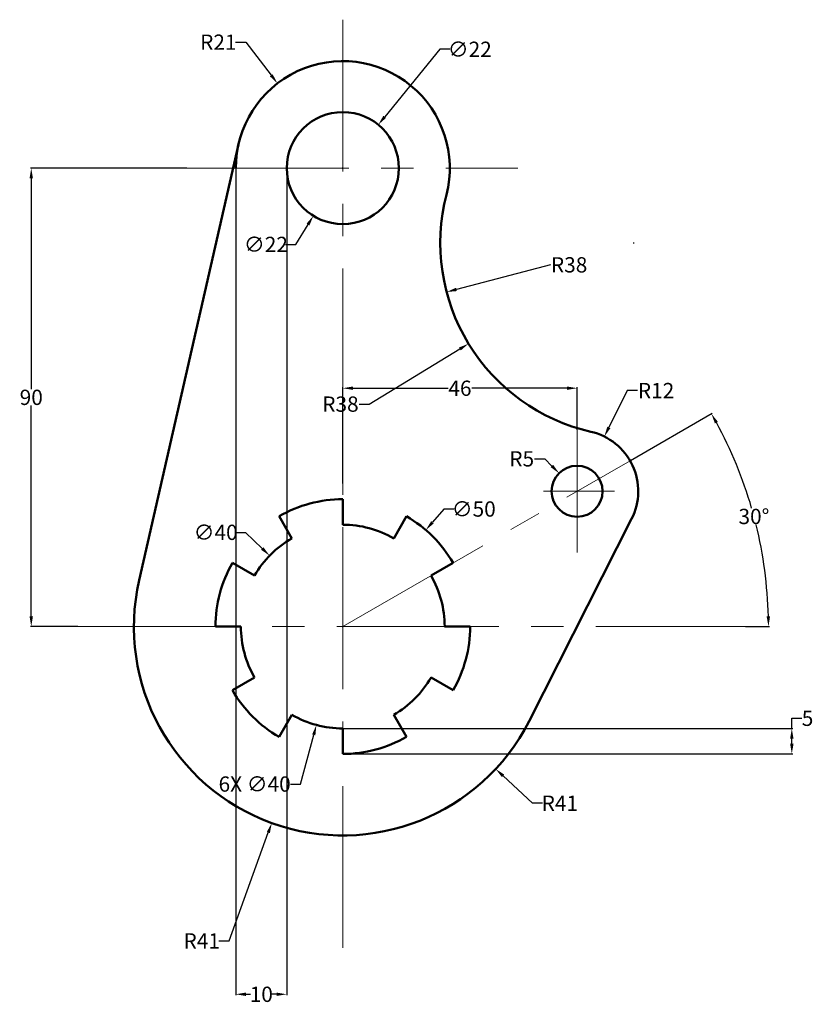
# Model space of a CAD drawing. Units: inches. Extents: x 93 to 249, y 22 to 215.
import ezdxf

# ---------------------------------------------------------------- set-up
doc = ezdxf.new("R2010")
doc.units = ezdxf.units.IN
doc.header["$MEASUREMENT"] = 0
doc.linetypes.add('CENTER', pattern=[50.8, 31.75, -6.35, 6.35, -6.35])
for name, color, linetype, lineweight in [('M-CNTR', 4, 'CENTER', 18), ('M-DIMS', 2, 'Continuous', 25), ('M-OUTL', 7, 'Continuous', 50)]:
    doc.layers.add(name, color=color, linetype=linetype, lineweight=lineweight)
doc.styles.get("Standard").update_dxf_attribs({"font": 'arial.ttf'})
doc.dimstyles.get("Standard").update_dxf_attribs({"dimtxt": 3, "dimasz": 2, "dimexe": 0.18, "dimexo": 0.0625, "dimgap": 0.09, "dimtad": 0, "dimtih": 1, "dimtoh": 1, "dimdec": 0, "dimzin": 0, "dimdsep": 46, "dimtxsty": 'Standard', "dimcen": 0.09, "dimadec": 0, "dimazin": 0, "dimtfac": 1, "dimtdec": 0, "dimtofl": 0, "dimtmove": 0, "dimatfit": 3, "dimfxl": 1, "dimtolj": 1, "dimtzin": 0, "dimarcsym": 0})

# ---------------------------------------------------------------- blocks, each defined once
blk = doc.blocks.new('*U1')
for p, q in [((6.25, -1.16), (6.25, 3.84)), ((-3.75, -3.84), (-6.25, 0.49))]:
    blk.add_line(p, q)
blk.add_arc((6.25, -21.16), 25, 90, 120)
blk = doc.blocks.new('*U2')
at = {"layer": 'M-OUTL', "color": 0, "linetype": 'ByBlock', "lineweight": -2, "transparency": 16777216}
blk.add_blockref('*U1', (150.02, 117.01), dxfattribs=at)
for p, rotation in [((171.47, 111.84), 300), ((134.82, 101.02), 59.99999999999996), ((177.72, 90.68), 239.9999999999999), ((141.07, 79.85), 119.9999999999999), ((162.52, 74.69), 180)]:
    blk.add_blockref('*U1', p, dxfattribs=dict(at, rotation=rotation))
blk = doc.blocks.new('*D3')
at = {"layer": 'Defpoints', "color": 0, "transparency": 16777216}
for p in [(212.66, 128.41), (238.56, 110.36), (104.32, 95.85), (156.27, 95.85), (235.29, 95.85)]:
    blk.add_point(p, dxfattribs=at)
at = {"layer": 'M-DIMS', "color": 0, "lineweight": -2, "transparency": 16777216}
for p, q in [((212.72, 128.44), (228.79, 137.72)), ((235.35, 95.85), (240.01, 95.85))]:
    blk.add_line(p, q, dxfattribs=at)
for start, end in [(16.1552, 28.6286), (1.3714, 13.851)]:
    blk.add_arc((156.27, 95.85), 83.56, start, end, dxfattribs=at)
at = {"layer": 'M-DIMS', "color": 0, "transparency": 16777216}
for points in [[(229.32, 135.72), (229.9, 136.05), (228.63, 137.63)], [(240.14, 97.85), (239.47, 97.84), (239.83, 95.85)]]:
    blk.add_solid(points, dxfattribs=at)
at = {"layer": 'M-DIMS', "color": 0, "transparency": 16777216, "insert": (236.98, 117.47), "char_height": 3, "attachment_point": 5}
blk.add_mtext('\\A1;30°', dxfattribs=at)
blk = doc.blocks.new('*D4')
at = {"layer": 'Defpoints', "color": 0, "transparency": 16777216}
for p in [(207.61, 133.15), (202.27, 122.41)]:
    blk.add_point(p, dxfattribs=at)
at = {"layer": 'M-DIMS', "color": 0, "lineweight": -2, "transparency": 16777216}
for p, q in [((212.1, 142.18), (208.5, 134.94)), ((214.1, 142.18), (212.1, 142.18)), ((202.18, 122.41), (202.36, 122.41)), ((202.27, 122.32), (202.27, 122.5))]:
    blk.add_line(p, q, dxfattribs=at)
at = {"layer": 'M-DIMS', "color": 0, "transparency": 16777216}
blk.add_solid([(208.2, 135.09), (208.8, 134.79), (207.61, 133.15)], dxfattribs=at)
at = {"layer": 'M-DIMS', "color": 0, "transparency": 16777216, "insert": (217.76, 142.18), "char_height": 3, "attachment_point": 5}
blk.add_mtext('\\A1;R12', dxfattribs=at)
blk = doc.blocks.new('*D5')
at = {"layer": 'Defpoints', "color": 0, "transparency": 16777216}
for p in [(198.74, 125.95), (202.27, 122.41)]:
    blk.add_point(p, dxfattribs=at)
at = {"layer": 'M-DIMS', "color": 0, "lineweight": -2, "transparency": 16777216}
for p, q in [((193.91, 128.78), (195.91, 128.78)), ((195.91, 128.78), (197.33, 127.36)), ((202.18, 122.41), (202.36, 122.41)), ((202.27, 122.32), (202.27, 122.5))]:
    blk.add_line(p, q, dxfattribs=at)
at = {"layer": 'M-DIMS', "color": 0, "transparency": 16777216}
blk.add_solid([(197.56, 127.6), (197.09, 127.13), (198.74, 125.95)], dxfattribs=at)
at = {"layer": 'M-DIMS', "color": 0, "transparency": 16777216, "insert": (191.39, 128.78), "char_height": 3, "attachment_point": 5}
blk.add_mtext('\\A1;R5', dxfattribs=at)
blk = doc.blocks.new('*D6')
at = {"layer": 'Defpoints', "color": 0, "transparency": 16777216}
for p in [(172.57, 114.8), (139.97, 76.89)]:
    blk.add_point(p, dxfattribs=at)
at = {"layer": 'M-DIMS', "color": 0, "lineweight": -2, "transparency": 16777216}
for p, q in [((176.12, 118.93), (173.87, 116.32)), ((178.12, 118.93), (176.12, 118.93)), ((156.18, 95.85), (156.36, 95.85)), ((156.27, 95.76), (156.27, 95.94))]:
    blk.add_line(p, q, dxfattribs=at)
at = {"layer": 'M-DIMS', "color": 0, "transparency": 16777216}
blk.add_solid([(173.62, 116.54), (174.13, 116.1), (172.57, 114.8)], dxfattribs=at)
at = {"layer": 'M-DIMS', "color": 0, "transparency": 16777216, "insert": (181.98, 118.93), "char_height": 3, "attachment_point": 5}
blk.add_mtext('\\A1;∅50', dxfattribs=at)
blk = doc.blocks.new('*D7')
at = {"layer": 'Defpoints', "color": 0, "transparency": 16777216}
for p in [(141.91, 109.77), (170.63, 81.93)]:
    blk.add_point(p, dxfattribs=at)
at = {"layer": 'M-DIMS', "color": 0, "lineweight": -2, "transparency": 16777216}
for p, q in [((135.19, 114.35), (137.19, 114.35)), ((137.19, 114.35), (140.47, 111.16)), ((156.18, 95.85), (156.36, 95.85)), ((156.27, 95.76), (156.27, 95.94))]:
    blk.add_line(p, q, dxfattribs=at)
at = {"layer": 'M-DIMS', "color": 0, "transparency": 16777216}
blk.add_solid([(140.71, 111.4), (140.24, 110.92), (141.91, 109.77)], dxfattribs=at)
at = {"layer": 'M-DIMS', "color": 0, "transparency": 16777216, "insert": (131.32, 114.35), "char_height": 3, "attachment_point": 5}
blk.add_mtext('\\A1;∅40', dxfattribs=at)
blk = doc.blocks.new('*D8')
at = {"layer": 'Defpoints', "color": 0, "transparency": 16777216}
for p in [(156.27, 142.64), (202.27, 134.41), (156.27, 123.89)]:
    blk.add_point(p, dxfattribs=at)
at = {"layer": 'M-DIMS', "color": 0, "lineweight": -2, "transparency": 16777216}
for p, q in [((156.27, 123.95), (156.27, 142.82)), ((158.27, 142.64), (176.97, 142.64)), ((200.27, 142.64), (181.57, 142.64)), ((202.27, 134.47), (202.27, 142.82))]:
    blk.add_line(p, q, dxfattribs=at)
at = {"layer": 'M-DIMS', "color": 0, "transparency": 16777216}
for points in [[(158.27, 142.98), (158.27, 142.31), (156.27, 142.64)], [(200.27, 142.98), (200.27, 142.31), (202.27, 142.64)]]:
    blk.add_solid(points, dxfattribs=at)
at = {"layer": 'M-DIMS', "color": 0, "transparency": 16777216, "insert": (179.27, 142.64), "char_height": 3, "attachment_point": 5}
blk.add_mtext('\\A1;46', dxfattribs=at)
blk = doc.blocks.new('*D9')
at = {"layer": 'Defpoints', "color": 0, "transparency": 16777216}
for p in [(213.41, 171.15), (176.65, 161.53)]:
    blk.add_point(p, dxfattribs=at)
at = {"layer": 'M-DIMS', "color": 0, "lineweight": -2, "transparency": 16777216}
blk.add_line((197.02, 166.86), (178.58, 162.04), dxfattribs=at)
at = {"layer": 'M-DIMS', "color": 0, "transparency": 16777216}
blk.add_solid([(178.5, 162.36), (178.67, 161.71), (176.65, 161.53)], dxfattribs=at)
at = {"layer": 'M-DIMS', "color": 0, "transparency": 16777216, "insert": (200.7, 166.86), "char_height": 3, "attachment_point": 5}
blk.add_mtext('\\A1;R38', dxfattribs=at)
blk = doc.blocks.new('*D10')
at = {"layer": 'Defpoints', "color": 0, "transparency": 16777216}
for p in [(156.27, 95.85), (186.27, 67.91)]:
    blk.add_point(p, dxfattribs=at)
at = {"layer": 'M-DIMS', "color": 0, "lineweight": -2, "transparency": 16777216}
for p, q in [((156.18, 95.85), (156.36, 95.85)), ((156.27, 95.76), (156.27, 95.94)), ((193.49, 61.18), (187.74, 66.54)), ((195.49, 61.18), (193.49, 61.18))]:
    blk.add_line(p, q, dxfattribs=at)
at = {"layer": 'M-DIMS', "color": 0, "transparency": 16777216}
blk.add_solid([(187.96, 66.79), (187.51, 66.3), (186.27, 67.91)], dxfattribs=at)
at = {"layer": 'M-DIMS', "color": 0, "transparency": 16777216, "insert": (198.88, 61.18), "char_height": 3, "attachment_point": 5}
blk.add_mtext('\\A1;R41', dxfattribs=at)
blk = doc.blocks.new('*D11')
at = {"layer": 'Defpoints', "color": 0, "transparency": 16777216}
for p in [(95.12, 185.85), (125.73, 185.85), (104.32, 95.85)]:
    blk.add_point(p, dxfattribs=at)
at = {"layer": 'M-DIMS', "color": 0, "lineweight": -2, "transparency": 16777216}
for p, q in [((125.67, 185.85), (94.94, 185.85)), ((95.12, 183.85), (95.12, 142.47)), ((95.12, 97.85), (95.12, 139.23)), ((104.26, 95.85), (94.94, 95.85))]:
    blk.add_line(p, q, dxfattribs=at)
at = {"layer": 'M-DIMS', "color": 0, "transparency": 16777216}
for points in [[(94.79, 183.85), (95.45, 183.85), (95.12, 185.85)], [(94.79, 97.85), (95.45, 97.85), (95.12, 95.85)]]:
    blk.add_solid(points, dxfattribs=at)
at = {"layer": 'M-DIMS', "color": 0, "transparency": 16777216, "insert": (95.12, 140.85), "char_height": 3, "attachment_point": 5}
blk.add_mtext('\\A1;90', dxfattribs=at)
blk = doc.blocks.new('*D12')
at = {"layer": 'Defpoints', "color": 0, "transparency": 16777216}
for p in [(143.45, 202.48), (156.27, 185.85)]:
    blk.add_point(p, dxfattribs=at)
at = {"layer": 'M-DIMS', "color": 0, "lineweight": -2, "transparency": 16777216}
for p, q in [((135.22, 210.57), (137.22, 210.57)), ((137.22, 210.57), (142.23, 204.07)), ((156.18, 185.85), (156.36, 185.85)), ((156.27, 185.76), (156.27, 185.94))]:
    blk.add_line(p, q, dxfattribs=at)
at = {"layer": 'M-DIMS', "color": 0, "transparency": 16777216}
blk.add_solid([(142.5, 204.27), (141.97, 203.86), (143.45, 202.48)], dxfattribs=at)
at = {"layer": 'M-DIMS', "color": 0, "transparency": 16777216, "insert": (131.84, 210.57), "char_height": 3, "attachment_point": 5}
blk.add_mtext('\\A1;R21', dxfattribs=at)
blk = doc.blocks.new('*D13')
at = {"layer": 'Defpoints', "color": 0, "transparency": 16777216}
for p in [(163.23, 194.36), (149.3, 177.33)]:
    blk.add_point(p, dxfattribs=at)
at = {"layer": 'M-DIMS', "color": 0, "lineweight": -2, "transparency": 16777216}
for p, q in [((175.34, 209.17), (164.5, 195.91)), ((177.34, 209.17), (175.34, 209.17)), ((156.18, 185.85), (156.36, 185.85)), ((156.27, 185.76), (156.27, 185.94))]:
    blk.add_line(p, q, dxfattribs=at)
at = {"layer": 'M-DIMS', "color": 0, "transparency": 16777216}
blk.add_solid([(164.24, 196.12), (164.76, 195.7), (163.23, 194.36)], dxfattribs=at)
at = {"layer": 'M-DIMS', "color": 0, "transparency": 16777216, "insert": (181.2, 209.17), "char_height": 3, "attachment_point": 5}
blk.add_mtext('\\A1;∅22', dxfattribs=at)
blk = doc.blocks.new('*D14')
at = {"layer": 'Defpoints', "color": 0, "transparency": 16777216}
for p in [(156.27, 75.85), (244.41, 75.85), (156.27, 70.85)]:
    blk.add_point(p, dxfattribs=at)
at = {"layer": 'M-DIMS', "color": 0, "lineweight": -2, "transparency": 16777216}
for p, q in [((244.41, 75.85), (244.41, 77.85)), ((244.41, 77.85), (246.41, 77.85)), ((156.33, 75.85), (244.59, 75.85)), ((244.41, 72.85), (244.41, 73.85)), ((156.33, 70.85), (244.59, 70.85))]:
    blk.add_line(p, q, dxfattribs=at)
at = {"layer": 'M-DIMS', "color": 0, "transparency": 16777216}
for points in [[(244.08, 73.85), (244.75, 73.85), (244.41, 75.85)], [(244.08, 72.85), (244.75, 72.85), (244.41, 70.85)]]:
    blk.add_solid(points, dxfattribs=at)
at = {"layer": 'M-DIMS', "color": 0, "transparency": 16777216, "insert": (247.5, 77.85), "char_height": 3, "attachment_point": 5}
blk.add_mtext('\\A1;5', dxfattribs=at)
blk = doc.blocks.new('*D15')
at = {"layer": 'Defpoints', "color": 0, "transparency": 16777216}
for p in [(135.27, 185.85), (145.27, 185.85), (145.27, 23.67)]:
    blk.add_point(p, dxfattribs=at)
at = {"layer": 'M-DIMS', "color": 0, "lineweight": -2, "transparency": 16777216}
for p, q in [((135.27, 185.79), (135.27, 23.49)), ((145.27, 185.79), (145.27, 23.49)), ((137.27, 23.67), (138.18, 23.67)), ((143.27, 23.67), (142.36, 23.67))]:
    blk.add_line(p, q, dxfattribs=at)
at = {"layer": 'M-DIMS', "color": 0, "transparency": 16777216}
for points in [[(137.27, 24.01), (137.27, 23.34), (135.27, 23.67)], [(143.27, 24.01), (143.27, 23.34), (145.27, 23.67)]]:
    blk.add_solid(points, dxfattribs=at)
at = {"layer": 'M-DIMS', "color": 0, "transparency": 16777216, "insert": (140.27, 23.67), "char_height": 3, "attachment_point": 5}
blk.add_mtext('\\A1;10', dxfattribs=at)
blk = doc.blocks.new('*D16')
at = {"layer": 'Defpoints', "color": 0, "transparency": 16777216}
for p in [(156.27, 95.85), (142.33, 57.29)]:
    blk.add_point(p, dxfattribs=at)
at = {"layer": 'M-DIMS', "color": 0, "lineweight": -2, "transparency": 16777216}
for p, q in [((156.18, 95.85), (156.36, 95.85)), ((156.27, 95.76), (156.27, 95.94)), ((133.97, 34.15), (141.65, 55.41)), ((131.97, 34.15), (133.97, 34.15))]:
    blk.add_line(p, q, dxfattribs=at)
at = {"layer": 'M-DIMS', "color": 0, "transparency": 16777216}
blk.add_solid([(141.34, 55.52), (141.96, 55.3), (142.33, 57.29)], dxfattribs=at)
at = {"layer": 'M-DIMS', "color": 0, "transparency": 16777216, "insert": (128.58, 34.15), "char_height": 3, "attachment_point": 5}
blk.add_mtext('\\A1;R41', dxfattribs=at)
blk = doc.blocks.new('*D17')
at = {"layer": 'Defpoints', "color": 0, "transparency": 16777216}
for p in [(213.41, 171.15), (180.96, 151.38)]:
    blk.add_point(p, dxfattribs=at)
at = {"layer": 'M-DIMS', "color": 0, "lineweight": -2, "transparency": 16777216}
for p, q in [((213.32, 171.15), (213.5, 171.15)), ((213.41, 171.06), (213.41, 171.24)), ((161.48, 139.52), (179.25, 150.34)), ((159.48, 139.52), (161.48, 139.52))]:
    blk.add_line(p, q, dxfattribs=at)
at = {"layer": 'M-DIMS', "color": 0, "transparency": 16777216}
blk.add_solid([(179.07, 150.62), (179.42, 150.05), (180.96, 151.38)], dxfattribs=at)
at = {"layer": 'M-DIMS', "color": 0, "transparency": 16777216, "insert": (155.81, 139.52), "char_height": 3, "attachment_point": 5}
blk.add_mtext('\\A1;R38', dxfattribs=at)
blk = doc.blocks.new('*D18')
at = {"layer": 'Defpoints', "color": 0, "transparency": 16777216}
for p in [(162.04, 195.21), (150.5, 176.48)]:
    blk.add_point(p, dxfattribs=at)
at = {"layer": 'M-DIMS', "color": 0, "lineweight": -2, "transparency": 16777216}
for p, q in [((156.18, 185.85), (156.36, 185.85)), ((156.27, 185.76), (156.27, 185.94)), ((147.03, 170.87), (149.45, 174.78)), ((145.03, 170.87), (147.03, 170.87))]:
    blk.add_line(p, q, dxfattribs=at)
at = {"layer": 'M-DIMS', "color": 0, "transparency": 16777216}
blk.add_solid([(149.16, 174.96), (149.73, 174.61), (150.5, 176.48)], dxfattribs=at)
at = {"layer": 'M-DIMS', "color": 0, "transparency": 16777216, "insert": (141.18, 170.87), "char_height": 3, "attachment_point": 5}
blk.add_mtext('\\A1;∅22', dxfattribs=at)
blk = doc.blocks.new('*D19')
at = {"layer": 'Defpoints', "color": 0, "transparency": 16777216}
for p in [(161.45, 115.17), (151.09, 76.53)]:
    blk.add_point(p, dxfattribs=at)
at = {"layer": 'M-DIMS', "color": 0, "lineweight": -2, "transparency": 16777216}
for p, q in [((156.18, 95.85), (156.36, 95.85)), ((156.27, 95.76), (156.27, 95.94)), ((147.98, 64.94), (150.57, 74.6)), ((145.98, 64.94), (147.98, 64.94))]:
    blk.add_line(p, q, dxfattribs=at)
at = {"layer": 'M-DIMS', "color": 0, "transparency": 16777216}
blk.add_solid([(150.25, 74.68), (150.89, 74.51), (151.09, 76.53)], dxfattribs=at)
at = {"layer": 'M-DIMS', "color": 0, "transparency": 16777216, "insert": (138.97, 64.94), "char_height": 3, "attachment_point": 5}
blk.add_mtext('\\A1;6X ∅40', dxfattribs=at)

msp = doc.modelspace()

# ---------------------------------------------------------------- linework, layer by layer
at = {"layer": 'M-CNTR'}
for p, q in [((156.27, 32.79), (156.27, 214.98)), ((125.73, 185.85), (190.62, 185.85)), ((202.27, 134.41), (202.27, 110.42)), ((156.27, 95.85), (212.66, 128.41)), ((195.65, 122.41), (209.62, 122.41)), ((104.32, 95.85), (235.29, 95.85))]:
    msp.add_line(p, q, dxfattribs=at)
at = {"layer": 'M-OUTL'}
for p, q in [((116.29, 104.96), (135.79, 190.51)), ((192.83, 77.29), (212.97, 116.97)), ((136.27, 95.85), (131.27, 95.85))]:
    msp.add_line(p, q, dxfattribs=at)
for centre, radius in [((156.27, 185.85), 11), ((202.27, 122.41), 5)]:
    msp.add_circle(centre, radius, dxfattribs=at)
for centre, radius, start, end in [((156.27, 185.85), 21, 345.574, 180), ((213.41, 171.15), 38, 165.574, 257.1268), ((202.27, 122.41), 12, 333.0911, 77.1268), ((156.27, 95.85), 20, 60, 90), ((156.27, 95.85), 20, 120, 150), ((156.27, 95.85), 41, 167.1604, 333.0911), ((156.27, 95.85), 20, 0, 30), ((156.27, 95.85), 20, 180, 210), ((156.27, 95.85), 20, 300, 330), ((156.27, 95.85), 20, 240, 270)]:
    msp.add_arc(centre, radius, start, end, dxfattribs=at)

# ---------------------------------------------------------------- block references
msp.add_blockref('*U2', (0, 0), dxfattribs=at)

# ---------------------------------------------------------------- dimensions: what is measured, and where the dimension line sits
at = {"layer": 'M-DIMS'}
for center, mpoint, override, picture, middle in [((156.27, 185.85), (143.45, 202.48), {"dimclrd": 0, "dimclre": 0, "dimclrt": 0}, '*D12', (131.84, 210.57)), ((213.41, 171.15), (180.96, 151.38), {"dimdec": 0, "dimlfac": 1, "dimrnd": 0, "dimzin": 0, "dimdsep": 46, "dimlunit": 2}, '*D17', (155.81, 139.52)), ((213.41, 171.15), (176.65, 161.53), {"dimclrd": 0, "dimclre": 0, "dimclrt": 0}, '*D9', (197.02, 166.86)), ((202.27, 122.41), (207.61, 133.15), {"dimclrd": 0, "dimclre": 0, "dimclrt": 0}, '*D4', (217.76, 142.18)), ((156.27, 95.85), (142.33, 57.29), {"dimdec": 0, "dimlfac": 1, "dimrnd": 0, "dimzin": 0, "dimdsep": 46, "dimlunit": 2}, '*D16', (128.58, 34.15)), ((156.27, 95.85), (186.27, 67.91), {"dimclrd": 0, "dimclre": 0, "dimclrt": 0}, '*D10', (198.88, 61.18))]:
    dim = msp.add_radius_dim(center=center, mpoint=mpoint, dimstyle='Standard', override=override, dxfattribs=at)
    dim.commit()
    dim.dimension.update_dxf_attribs({"geometry": picture, "text_midpoint": middle, "dimtype": 164})
for p1, p2, override, picture, middle in [((149.3, 177.33), (163.23, 194.36), {"dimclrd": 0, "dimclre": 0, "dimclrt": 0}, '*D13', (181.2, 209.17)), ((162.04, 195.21), (150.5, 176.48), {"dimdec": 0, "dimlfac": 1, "dimrnd": 0, "dimzin": 0, "dimdsep": 46, "dimlunit": 2}, '*D18', (141.18, 170.87)), ((139.97, 76.89), (172.57, 114.8), {"dimclrd": 0, "dimclre": 0, "dimclrt": 0}, '*D6', (181.98, 118.93)), ((170.63, 81.93), (141.91, 109.77), {"dimclrd": 0, "dimclre": 0, "dimclrt": 0}, '*D7', (131.32, 114.35))]:
    dim = msp.add_diameter_dim_2p(p1=p1, p2=p2, dimstyle='Standard', override=override, dxfattribs=at)
    dim.commit()
    dim.dimension.update_dxf_attribs({"geometry": picture, "text_midpoint": middle, "dimtype": 163})
for base, p1, p2, override, picture, middle in [((95.12, 185.85), (104.32, 95.85), (125.73, 185.85), {"dimclrd": 0, "dimclre": 0, "dimclrt": 0}, '*D11', (95.12, 140.85)), ((244.41, 75.85), (156.27, 70.85), (156.27, 75.85), {"dimdec": 0, "dimlfac": 1, "dimrnd": 0, "dimzin": 0, "dimdsep": 46, "dimlunit": 2}, '*D14', (247.5, 77.85))]:
    dim = msp.add_linear_dim(base=base, p1=p1, p2=p2, angle=90, dimstyle='Standard', override=override, dxfattribs=at)
    dim.commit()
    dim.dimension.update_dxf_attribs({"geometry": picture, "text_midpoint": middle})
for base, p1, p2, override, picture, middle in [((145.27, 23.67), (135.27, 185.85), (145.27, 185.85), {"dimdec": 0, "dimlfac": 1, "dimrnd": 0, "dimzin": 0, "dimdsep": 46, "dimlunit": 2}, '*D15', (140.27, 23.67)), ((156.27, 142.64), (202.27, 134.41), (156.27, 123.89), {"dimclrd": 0, "dimclre": 0, "dimclrt": 0}, '*D8', (179.27, 142.64))]:
    dim = msp.add_linear_dim(base=base, p1=p1, p2=p2, dimstyle='Standard', override=override, dxfattribs=at)
    dim.commit()
    dim.dimension.update_dxf_attribs({"geometry": picture, "text_midpoint": middle})
dim = msp.add_angular_dim_2l(base=(238.56, 110.36), line1=((104.32, 95.85), (235.29, 95.85)), line2=((156.27, 95.85), (212.66, 128.41)), dimstyle='Standard', override={"dimclrd": 0, "dimclre": 0, "dimclrt": 0}, dxfattribs=at)
dim.commit()
dim.dimension.update_dxf_attribs({"geometry": '*D3', "text_midpoint": (236.98, 117.47)})
dim = msp.add_radius_dim(center=(202.27, 122.41), mpoint=(198.74, 125.95), dimstyle='Standard', override={"dimclrd": 0, "dimclre": 0, "dimclrt": 0}, dxfattribs=at)
dim.commit()
dim.dimension.update_dxf_attribs({"geometry": '*D5', "text_midpoint": (191.39, 128.78)})
dim = msp.add_diameter_dim_2p(p1=(161.45, 115.17), p2=(151.09, 76.53), text='6X <>', dimstyle='Standard', override={"dimdec": 0, "dimlfac": 1, "dimrnd": 0, "dimzin": 0, "dimdsep": 46, "dimlunit": 2}, dxfattribs=at)
dim.commit()
dim.dimension.update_dxf_attribs({"geometry": '*D19', "text_midpoint": (138.97, 64.94), "dimtype": 163})

doc.saveas('drawing.dxf')
